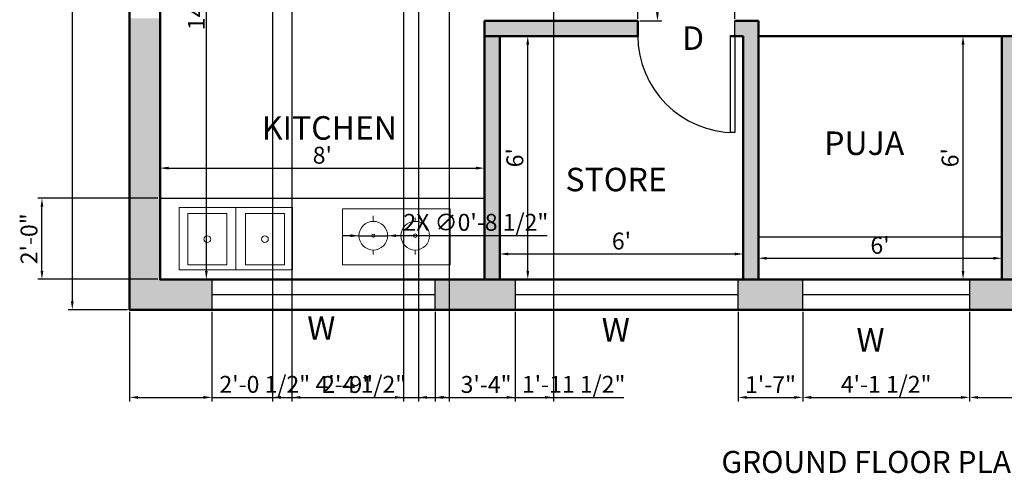
# Model space of a CAD drawing. Units: inches. Extents: x 2168 to 2706, y 2255 to 2760.
# Tile 1 of 4: x 2172 to 2463, y 2255 to 2389. Entities that reach past the tile are written whole.
import ezdxf

# ---------------------------------------------------------------- set-up
doc = ezdxf.new("R2010")
doc.units = ezdxf.units.IN
for name, color, linetype, lineweight in [('A-ANNO-DIMS', 220, 'Continuous', 18), ('A-ANNO-TEXT', 220, 'Continuous', 25), ('A-AREA-IDEN', 220, 'Continuous', 25), ('A-EQPM', 112, 'Continuous', 18), ('A-FLOR-CASE', 112, 'Continuous', 25), ('A-FLOR-FIXT', 9, 'Continuous', 18), ('A-WALL-PATT', 140, 'Continuous', 13), ('DOOR', 30, 'Continuous', 25), ('WALL', 140, 'Continuous', 50), ('WINDOW', 200, 'Continuous', 25)]:
    doc.layers.add(name, color=color, linetype=linetype, lineweight=lineweight)
doc.styles.get("Standard").update_dxf_attribs({"font": 'arial.ttf'})
doc.dimstyles.new('ISO-25', dxfattribs={"dimtxt": 5, "dimasz": 2.5, "dimexe": 1.25, "dimexo": 0.625, "dimtad": 1, "dimlunit": 4, "dimtxsty": 'Standard', "dimcen": 2.5, "dimadec": 0, "dimazin": 0, "dimtfac": 1, "dimtmove": 0, "dimatfit": 3, "dimfxl": 1, "dimarcsym": 0})

# ---------------------------------------------------------------- blocks, each defined once
blk = doc.blocks.new('*U2')
for p, q in [((0, 0), (0, -6)), ((40, 0), (40, -6))]:
    blk.add_line(p, q)
blk.add_lwpolyline([(0, 0), (0, 40), (1.75, 40), (1.75, 0)], close=True)
blk.add_arc((0, 0), 40, 0, 90)
blk = doc.blocks.new('*D11')
at = {"layer": 'A-ANNO-DIMS', "color": 0, "lineweight": -2, "transparency": 16777216}
for p, q in [((2213.72, 2312.97), (2213.72, 2346.52)), ((2216.22, 2345.27), (2307.22, 2345.27)), ((2309.72, 2312.97), (2309.72, 2346.52))]:
    blk.add_line(p, q, dxfattribs=at)
at = {"layer": 'A-ANNO-DIMS', "color": 0, "transparency": 16777216}
for points in [[(2216.22, 2345.69), (2216.22, 2344.85), (2213.72, 2345.27)], [(2307.22, 2345.69), (2307.22, 2344.85), (2309.72, 2345.27)]]:
    blk.add_solid(points, dxfattribs=at)
at = {"layer": 'Defpoints', "color": 0, "transparency": 16777216}
for p in [(2309.72, 2345.27), (2213.72, 2312.35), (2309.72, 2312.35)]:
    blk.add_point(p, dxfattribs=at)
at = {"layer": 'A-ANNO-DIMS', "color": 0, "transparency": 16777216, "insert": (2261.72, 2348.45), "char_height": 5, "attachment_point": 5}
blk.add_mtext("8'", dxfattribs=at)
blk = doc.blocks.new('*D12')
at = {"layer": 'A-ANNO-DIMS', "color": 0, "lineweight": -2, "transparency": 16777216}
for p, q in [((2314.22, 2312.97), (2314.22, 2321.11)), ((2316.72, 2319.86), (2383.72, 2319.86)), ((2386.22, 2312.97), (2386.22, 2321.11))]:
    blk.add_line(p, q, dxfattribs=at)
at = {"layer": 'A-ANNO-DIMS', "color": 0, "transparency": 16777216}
for points in [[(2316.72, 2320.27), (2316.72, 2319.44), (2314.22, 2319.86)], [(2383.72, 2320.27), (2383.72, 2319.44), (2386.22, 2319.86)]]:
    blk.add_solid(points, dxfattribs=at)
at = {"layer": 'Defpoints', "color": 0, "transparency": 16777216}
for p in [(2386.22, 2319.86), (2314.22, 2312.35), (2386.22, 2312.35)]:
    blk.add_point(p, dxfattribs=at)
at = {"layer": 'A-ANNO-DIMS', "color": 0, "transparency": 16777216, "insert": (2350.22, 2323.04), "char_height": 5, "attachment_point": 5}
blk.add_mtext("6'", dxfattribs=at)
blk = doc.blocks.new('*D13')
at = {"layer": 'A-ANNO-DIMS', "color": 0, "lineweight": -2, "transparency": 16777216}
for p, q in [((2390.72, 2312.97), (2390.72, 2319.84)), ((2462.72, 2312.97), (2462.72, 2319.84)), ((2393.22, 2318.59), (2460.22, 2318.59))]:
    blk.add_line(p, q, dxfattribs=at)
at = {"layer": 'A-ANNO-DIMS', "color": 0, "transparency": 16777216}
for points in [[(2393.22, 2319.01), (2393.22, 2318.17), (2390.72, 2318.59)], [(2460.22, 2319.01), (2460.22, 2318.17), (2462.72, 2318.59)]]:
    blk.add_solid(points, dxfattribs=at)
at = {"layer": 'Defpoints', "color": 0, "transparency": 16777216}
for p in [(2462.72, 2318.59), (2390.72, 2312.35), (2462.72, 2312.35)]:
    blk.add_point(p, dxfattribs=at)
at = {"layer": 'A-ANNO-DIMS', "color": 0, "transparency": 16777216, "insert": (2426.72, 2321.77), "char_height": 5, "attachment_point": 5}
blk.add_mtext("6'", dxfattribs=at)
blk = doc.blocks.new('*D24')
at = {"layer": 'A-ANNO-DIMS', "color": 0, "lineweight": -2, "transparency": 16777216}
for p, q in [((2355.67, 2565.85), (2362.12, 2565.85)), ((2360.87, 2391.35), (2360.87, 2563.35)), ((2355.67, 2388.85), (2362.12, 2388.85))]:
    blk.add_line(p, q, dxfattribs=at)
at = {"layer": 'A-ANNO-DIMS', "color": 0, "transparency": 16777216}
for points in [[(2360.45, 2563.35), (2361.28, 2563.35), (2360.87, 2565.85)], [(2360.45, 2391.35), (2361.28, 2391.35), (2360.87, 2388.85)]]:
    blk.add_solid(points, dxfattribs=at)
at = {"layer": 'Defpoints', "color": 0, "transparency": 16777216}
for p in [(2355.04, 2565.85), (2360.87, 2565.85), (2355.04, 2388.85)]:
    blk.add_point(p, dxfattribs=at)
at = {"layer": 'A-ANNO-DIMS', "color": 0, "transparency": 16777216, "insert": (2357.69, 2477.35), "char_height": 5, "attachment_point": 5, "rotation": 90}
blk.add_mtext('14\'-9"', dxfattribs=at)
blk = doc.blocks.new('*D26')
at = {"layer": 'A-ANNO-DIMS', "color": 0, "lineweight": -2, "transparency": 16777216}
for p, q in [((2462.1, 2384.35), (2450.03, 2384.35)), ((2451.28, 2314.85), (2451.28, 2381.85)), ((2462.1, 2312.35), (2450.03, 2312.35))]:
    blk.add_line(p, q, dxfattribs=at)
at = {"layer": 'A-ANNO-DIMS', "color": 0, "transparency": 16777216}
for points in [[(2450.87, 2381.85), (2451.7, 2381.85), (2451.28, 2384.35)], [(2450.87, 2314.85), (2451.7, 2314.85), (2451.28, 2312.35)]]:
    blk.add_solid(points, dxfattribs=at)
at = {"layer": 'Defpoints', "color": 0, "transparency": 16777216}
for p in [(2451.28, 2384.35), (2462.72, 2384.35), (2462.72, 2312.35)]:
    blk.add_point(p, dxfattribs=at)
at = {"layer": 'A-ANNO-DIMS', "color": 0, "transparency": 16777216, "insert": (2448.1, 2348.35), "char_height": 5, "attachment_point": 5, "rotation": 90}
blk.add_mtext("6'", dxfattribs=at)
blk = doc.blocks.new('*D27')
at = {"layer": 'A-ANNO-DIMS', "color": 0, "lineweight": -2, "transparency": 16777216}
for p, q in [((2314.85, 2384.35), (2323.75, 2384.35)), ((2322.5, 2314.85), (2322.5, 2381.85)), ((2314.85, 2312.35), (2323.75, 2312.35))]:
    blk.add_line(p, q, dxfattribs=at)
at = {"layer": 'A-ANNO-DIMS', "color": 0, "transparency": 16777216}
for points in [[(2322.09, 2381.85), (2322.92, 2381.85), (2322.5, 2384.35)], [(2322.09, 2314.85), (2322.92, 2314.85), (2322.5, 2312.35)]]:
    blk.add_solid(points, dxfattribs=at)
at = {"layer": 'Defpoints', "color": 0, "transparency": 16777216}
for p in [(2314.22, 2384.35), (2322.5, 2384.35), (2314.22, 2312.35)]:
    blk.add_point(p, dxfattribs=at)
at = {"layer": 'A-ANNO-DIMS', "color": 0, "transparency": 16777216, "insert": (2319.33, 2348.35), "char_height": 5, "attachment_point": 5, "rotation": 90}
blk.add_mtext("6'", dxfattribs=at)
blk = doc.blocks.new('*D28')
at = {"layer": 'A-ANNO-DIMS', "color": 0, "lineweight": -2, "transparency": 16777216}
for p, q in [((2214.35, 2482.49), (2228.66, 2482.49)), ((2227.41, 2314.85), (2227.41, 2479.99)), ((2214.35, 2312.35), (2228.66, 2312.35))]:
    blk.add_line(p, q, dxfattribs=at)
at = {"layer": 'A-ANNO-DIMS', "color": 0, "transparency": 16777216}
for points in [[(2227, 2479.99), (2227.83, 2479.99), (2227.41, 2482.49)], [(2227, 2314.85), (2227.83, 2314.85), (2227.41, 2312.35)]]:
    blk.add_solid(points, dxfattribs=at)
at = {"layer": 'Defpoints', "color": 0, "transparency": 16777216}
for p in [(2213.72, 2482.49), (2227.41, 2482.49), (2213.72, 2312.35)]:
    blk.add_point(p, dxfattribs=at)
at = {"layer": 'A-ANNO-DIMS', "color": 0, "transparency": 16777216, "insert": (2220.94, 2397.42), "char_height": 5, "attachment_point": 5, "rotation": 90}
blk.add_mtext('14\'-2{\\H1x;\\S1/4;}"', dxfattribs=at)
blk = doc.blocks.new('*D30')
at = {"layer": 'A-ANNO-DIMS', "color": 0, "lineweight": -2, "transparency": 16777216}
for p, q in [((2204.1, 2723.35), (2186.49, 2723.35)), ((2187.74, 2720.85), (2187.74, 2305.85)), ((2204.1, 2303.35), (2186.49, 2303.35))]:
    blk.add_line(p, q, dxfattribs=at)
at = {"layer": 'A-ANNO-DIMS', "color": 0, "transparency": 16777216}
for points in [[(2187.33, 2720.85), (2188.16, 2720.85), (2187.74, 2723.35)], [(2187.33, 2305.85), (2188.16, 2305.85), (2187.74, 2303.35)]]:
    blk.add_solid(points, dxfattribs=at)
at = {"layer": 'Defpoints', "color": 0, "transparency": 16777216}
for p in [(2204.72, 2723.35), (2187.74, 2303.35), (2204.72, 2303.35)]:
    blk.add_point(p, dxfattribs=at)
at = {"layer": 'A-ANNO-DIMS', "color": 0, "transparency": 16777216, "insert": (2184.56, 2513.35), "char_height": 5, "attachment_point": 5, "rotation": 90}
blk.add_mtext("35'", dxfattribs=at)
blk = doc.blocks.new('WIN-66IN')
blk.add_line((0, 0), (66.01, 0))
blk.add_lwpolyline([(0, -4.5), (66.01, -4.5), (66.01, 4.5), (0, 4.5)], close=True)
blk = doc.blocks.new('*D49')
at = {"layer": 'A-ANNO-DIMS', "color": 0, "lineweight": -2, "transparency": 16777216}
for p, q in [((2355.04, 2389.47), (2355.04, 2750.55)), ((2383.78, 2389.47), (2383.78, 2750.55)), ((2357.54, 2749.3), (2381.28, 2749.3))]:
    blk.add_line(p, q, dxfattribs=at)
at = {"layer": 'A-ANNO-DIMS', "color": 0, "transparency": 16777216}
for points in [[(2357.54, 2749.71), (2357.54, 2748.88), (2355.04, 2749.3)], [(2381.28, 2749.71), (2381.28, 2748.88), (2383.78, 2749.3)]]:
    blk.add_solid(points, dxfattribs=at)
at = {"layer": 'Defpoints', "color": 0, "transparency": 16777216}
for p in [(2383.78, 2749.3), (2355.04, 2388.85), (2383.78, 2388.85)]:
    blk.add_point(p, dxfattribs=at)
at = {"layer": 'A-ANNO-DIMS', "color": 0, "transparency": 16777216, "insert": (2369.41, 2752.51), "char_height": 5, "attachment_point": 5}
blk.add_mtext('2\'-4 1/2"', dxfattribs=at)
blk = doc.blocks.new('*D54')
at = {"layer": 'A-ANNO-DIMS', "color": 0, "lineweight": -2, "transparency": 16777216}
for p, q in [((2246.96, 2425.79), (2246.96, 2276.15)), ((2299.27, 2425.79), (2299.27, 2276.15)), ((2249.46, 2277.4), (2296.77, 2277.4))]:
    blk.add_line(p, q, dxfattribs=at)
at = {"layer": 'A-ANNO-DIMS', "color": 0, "transparency": 16777216}
for points in [[(2249.46, 2277.81), (2249.46, 2276.98), (2246.96, 2277.4)], [(2296.77, 2277.81), (2296.77, 2276.98), (2299.27, 2277.4)]]:
    blk.add_solid(points, dxfattribs=at)
at = {"layer": 'Defpoints', "color": 0, "transparency": 16777216}
for p in [(2246.96, 2426.42), (2299.27, 2426.42), (2299.27, 2277.4)]:
    blk.add_point(p, dxfattribs=at)
at = {"layer": 'A-ANNO-DIMS', "color": 0, "transparency": 16777216, "insert": (2273.11, 2280.61), "char_height": 5, "attachment_point": 5}
blk.add_mtext('4\'-4 1/2"', dxfattribs=at)
blk = doc.blocks.new('*D56')
at = {"layer": 'A-ANNO-DIMS', "color": 0, "lineweight": -2, "transparency": 16777216}
for p, q in [((2213.1, 2336.35), (2177.52, 2336.35)), ((2178.77, 2314.85), (2178.77, 2333.85)), ((2213.1, 2312.35), (2177.52, 2312.35))]:
    blk.add_line(p, q, dxfattribs=at)
at = {"layer": 'A-ANNO-DIMS', "color": 0, "transparency": 16777216}
for points in [[(2178.36, 2333.85), (2179.19, 2333.85), (2178.77, 2336.35)], [(2178.36, 2314.85), (2179.19, 2314.85), (2178.77, 2312.35)]]:
    blk.add_solid(points, dxfattribs=at)
at = {"layer": 'Defpoints', "color": 0, "transparency": 16777216}
for p in [(2178.77, 2336.35), (2213.72, 2336.35), (2213.72, 2312.35)]:
    blk.add_point(p, dxfattribs=at)
at = {"layer": 'A-ANNO-DIMS', "color": 0, "transparency": 16777216, "insert": (2175.6, 2324.35), "char_height": 5, "attachment_point": 5, "rotation": 90}
blk.add_mtext('2\'-0"', dxfattribs=at)
blk = doc.blocks.new('*D57')
at = {"layer": 'A-ANNO-DIMS', "color": 0, "lineweight": -2, "transparency": 16777216}
for p, q in [((2204.72, 2302.72), (2204.72, 2276.15)), ((2229.06, 2302.72), (2229.06, 2276.15)), ((2207.22, 2277.4), (2226.56, 2277.4)), ((2229.06, 2277.4), (2257.84, 2277.4))]:
    blk.add_line(p, q, dxfattribs=at)
at = {"layer": 'A-ANNO-DIMS', "color": 0, "transparency": 16777216}
for points in [[(2207.22, 2277.81), (2207.22, 2276.98), (2204.72, 2277.4)], [(2226.56, 2277.81), (2226.56, 2276.98), (2229.06, 2277.4)]]:
    blk.add_solid(points, dxfattribs=at)
at = {"layer": 'Defpoints', "color": 0, "transparency": 16777216}
for p in [(2204.72, 2303.35), (2229.06, 2303.35), (2229.06, 2277.4)]:
    blk.add_point(p, dxfattribs=at)
at = {"layer": 'A-ANNO-DIMS', "color": 0, "transparency": 16777216, "insert": (2244.7, 2280.61), "char_height": 5, "attachment_point": 5}
blk.add_mtext('2\'-0 1/2"', dxfattribs=at)
blk = doc.blocks.new('*D58')
at = {"layer": 'A-ANNO-DIMS', "color": 0, "lineweight": -2, "transparency": 16777216}
for p, q in [((2295.07, 2302.72), (2295.07, 2276.15)), ((2318.77, 2302.72), (2318.77, 2276.15)), ((2297.57, 2277.4), (2316.27, 2277.4)), ((2318.77, 2277.4), (2350.88, 2277.4))]:
    blk.add_line(p, q, dxfattribs=at)
at = {"layer": 'A-ANNO-DIMS', "color": 0, "transparency": 16777216}
for points in [[(2297.57, 2277.81), (2297.57, 2276.98), (2295.07, 2277.4)], [(2316.27, 2277.81), (2316.27, 2276.98), (2318.77, 2277.4)]]:
    blk.add_solid(points, dxfattribs=at)
at = {"layer": 'Defpoints', "color": 0, "transparency": 16777216}
for p in [(2295.07, 2303.35), (2318.77, 2303.35), (2318.77, 2277.4)]:
    blk.add_point(p, dxfattribs=at)
at = {"layer": 'A-ANNO-DIMS', "color": 0, "transparency": 16777216, "insert": (2336.08, 2280.61), "char_height": 5, "attachment_point": 5}
blk.add_mtext('1\'-11 1/2"', dxfattribs=at)
blk = doc.blocks.new('*D59')
at = {"layer": 'A-ANNO-DIMS', "color": 0, "lineweight": -2, "transparency": 16777216}
for p, q in [((2384.78, 2302.72), (2384.78, 2276.15)), ((2403.85, 2302.72), (2403.85, 2276.15)), ((2387.28, 2277.4), (2401.35, 2277.4))]:
    blk.add_line(p, q, dxfattribs=at)
at = {"layer": 'A-ANNO-DIMS', "color": 0, "transparency": 16777216}
for points in [[(2387.28, 2277.81), (2387.28, 2276.98), (2384.78, 2277.4)], [(2401.35, 2277.81), (2401.35, 2276.98), (2403.85, 2277.4)]]:
    blk.add_solid(points, dxfattribs=at)
at = {"layer": 'Defpoints', "color": 0, "transparency": 16777216}
for p in [(2384.78, 2303.35), (2403.85, 2303.35), (2403.85, 2277.4)]:
    blk.add_point(p, dxfattribs=at)
at = {"layer": 'A-ANNO-DIMS', "color": 0, "transparency": 16777216, "insert": (2394.32, 2280.53), "char_height": 5, "attachment_point": 5}
blk.add_mtext('1\'-7"', dxfattribs=at)
blk = doc.blocks.new('*D60')
at = {"layer": 'A-ANNO-DIMS', "color": 0, "lineweight": -2, "transparency": 16777216}
for p, q in [((2403.85, 2302.72), (2403.85, 2276.15)), ((2453.21, 2302.72), (2453.21, 2276.15)), ((2406.35, 2277.4), (2450.71, 2277.4))]:
    blk.add_line(p, q, dxfattribs=at)
at = {"layer": 'A-ANNO-DIMS', "color": 0, "transparency": 16777216}
for points in [[(2406.35, 2277.81), (2406.35, 2276.98), (2403.85, 2277.4)], [(2450.71, 2277.81), (2450.71, 2276.98), (2453.21, 2277.4)]]:
    blk.add_solid(points, dxfattribs=at)
at = {"layer": 'Defpoints', "color": 0, "transparency": 16777216}
for p in [(2403.85, 2303.35), (2453.21, 2303.35), (2453.21, 2277.4)]:
    blk.add_point(p, dxfattribs=at)
at = {"layer": 'A-ANNO-DIMS', "color": 0, "transparency": 16777216, "insert": (2428.53, 2280.61), "char_height": 5, "attachment_point": 5}
blk.add_mtext('4\'-1 1/2"', dxfattribs=at)
blk = doc.blocks.new('*D61')
at = {"layer": 'A-ANNO-DIMS', "color": 0, "lineweight": -2, "transparency": 16777216}
for p, q in [((2453.21, 2302.72), (2453.21, 2276.15)), ((2493.42, 2302.72), (2493.42, 2276.15)), ((2455.71, 2277.4), (2490.92, 2277.4))]:
    blk.add_line(p, q, dxfattribs=at)
at = {"layer": 'A-ANNO-DIMS', "color": 0, "transparency": 16777216}
for points in [[(2455.71, 2277.81), (2455.71, 2276.98), (2453.21, 2277.4)], [(2490.92, 2277.81), (2490.92, 2276.98), (2493.42, 2277.4)]]:
    blk.add_solid(points, dxfattribs=at)
at = {"layer": 'Defpoints', "color": 0, "transparency": 16777216}
for p in [(2453.21, 2303.35), (2493.42, 2303.35), (2493.42, 2277.4)]:
    blk.add_point(p, dxfattribs=at)
at = {"layer": 'A-ANNO-DIMS', "color": 0, "transparency": 16777216, "insert": (2473.31, 2280.58), "char_height": 5, "attachment_point": 5}
blk.add_mtext('3\'-4"', dxfattribs=at)
blk = doc.blocks.new('*D64')
at = {"layer": 'A-ANNO-DIMS', "color": 0, "lineweight": -2, "transparency": 16777216}
for p, q in [((2290.22, 2713.72), (2290.22, 2276.15)), ((2330.12, 2713.72), (2330.12, 2276.15)), ((2292.72, 2277.4), (2327.62, 2277.4))]:
    blk.add_line(p, q, dxfattribs=at)
at = {"layer": 'A-ANNO-DIMS', "color": 0, "transparency": 16777216}
for points in [[(2292.72, 2277.81), (2292.72, 2276.98), (2290.22, 2277.4)], [(2327.62, 2277.81), (2327.62, 2276.98), (2330.12, 2277.4)]]:
    blk.add_solid(points, dxfattribs=at)
at = {"layer": 'Defpoints', "color": 0, "transparency": 16777216}
for p in [(2290.22, 2714.35), (2330.12, 2714.35), (2330.12, 2277.4)]:
    blk.add_point(p, dxfattribs=at)
at = {"layer": 'A-ANNO-DIMS', "color": 0, "transparency": 16777216, "insert": (2310.17, 2280.58), "char_height": 5, "attachment_point": 5}
blk.add_mtext('3\'-4"', dxfattribs=at)
blk = doc.blocks.new('*D76')
at = {"layer": 'A-ANNO-DIMS', "color": 0, "lineweight": -2, "transparency": 16777216}
for p, q in [((2252.72, 2623.46), (2252.72, 2276.15)), ((2285.72, 2612.95), (2285.72, 2276.15)), ((2255.22, 2277.4), (2283.22, 2277.4))]:
    blk.add_line(p, q, dxfattribs=at)
at = {"layer": 'A-ANNO-DIMS', "color": 0, "transparency": 16777216}
for points in [[(2255.22, 2277.81), (2255.22, 2276.98), (2252.72, 2277.4)], [(2283.22, 2277.81), (2283.22, 2276.98), (2285.72, 2277.4)]]:
    blk.add_solid(points, dxfattribs=at)
at = {"layer": 'Defpoints', "color": 0, "transparency": 16777216}
for p in [(2252.72, 2624.08), (2285.72, 2613.58), (2285.72, 2277.4)]:
    blk.add_point(p, dxfattribs=at)
at = {"layer": 'A-ANNO-DIMS', "color": 0, "transparency": 16777216, "insert": (2269.22, 2280.57), "char_height": 5, "attachment_point": 5}
blk.add_mtext('2\'-9"', dxfattribs=at)
blk = doc.blocks.new('*D78')
at = {"layer": 'A-ANNO-DIMS', "color": 0, "lineweight": -2, "transparency": 16777216}
for p, q in [((2270.05, 2325.26), (2267.55, 2325.26)), ((2272.55, 2325.26), (2281.04, 2325.26)), ((2328.24, 2325.26), (2283.54, 2325.26))]:
    blk.add_line(p, q, dxfattribs=at)
at = {"layer": 'A-ANNO-DIMS', "color": 0, "transparency": 16777216}
for points in [[(2270.05, 2325.68), (2270.05, 2324.84), (2272.55, 2325.26)], [(2283.54, 2325.68), (2283.54, 2324.84), (2281.04, 2325.26)]]:
    blk.add_solid(points, dxfattribs=at)
at = {"layer": 'Defpoints', "color": 0, "transparency": 16777216}
for p in [(2272.55, 2325.26), (2281.04, 2325.26)]:
    blk.add_point(p, dxfattribs=at)
at = {"layer": 'A-ANNO-DIMS', "color": 0, "transparency": 16777216, "insert": (2307.14, 2328.58), "char_height": 5, "attachment_point": 5, "rotation": 359.9965}
blk.add_mtext('2X ∅0\'-8 1/2"', dxfattribs=at)

msp = doc.modelspace()

# ---------------------------------------------------------------- hatches: boundary and pattern name
at = {"layer": 'A-WALL-PATT'}
h = msp.add_hatch(color=256, dxfattribs=at)
h.dxf.hatch_style = 1
h.paths.add_polyline_path([(2330.12, 2723.347), (2204.724, 2723.347), (2204.724, 2662.147), (2213.724, 2662.147), (2213.724, 2714.347), (2285.724, 2714.347), (2330.12, 2714.347)])
h.paths.add_polyline_path([(2496.542, 2723.347), (2396.128, 2723.347), (2396.128, 2714.347), (2434.224, 2714.347), (2496.542, 2714.347)])
h.paths.add_polyline_path([(2624.724, 2723.347), (2562.55, 2723.347), (2562.55, 2714.347), (2615.724, 2714.347), (2615.724, 2545.448), (2624.724, 2545.448)])
h.paths.add_polyline_path([(2438.724, 2714.347), (2434.224, 2714.347), (2434.224, 2570.347), (2426.591, 2570.347), (2426.591, 2565.847), (2438.724, 2565.847), (2444.149, 2565.847), (2444.149, 2570.347), (2438.724, 2570.347)])
h.paths.add_polyline_path([(2290.224, 2668.023), (2285.724, 2668.023), (2285.724, 2570.347), (2213.724, 2570.347), (2213.724, 2565.847), (2290.224, 2565.847), (2386.591, 2565.847), (2386.591, 2570.347), (2290.224, 2570.347)])
h.paths.add_polyline_path([(2514.678, 2570.347), (2514.678, 2630.11), (2560.439, 2630.11), (2560.439, 2570.347)], flags=16)
h.paths.add_polyline_path([(2517.528, 2574.595), (2517.528, 2583.399), (2536.063, 2583.399), (2536.063, 2574.595)], flags=0)
h.paths.add_polyline_path([(2523.909, 2586.89), (2514.678, 2597.212), (2518.822, 2600.918)], flags=0)
h.paths.add_polyline_path([(2538.189, 2574.595), (2538.189, 2583.399), (2556.724, 2583.399), (2556.724, 2574.595)], flags=0)
h.paths.add_polyline_path([(2560.439, 2630.11), (2560.439, 2570.347), (2514.678, 2570.347), (2514.678, 2630.11)])
h.paths.add_polyline_path([(2213.724, 2389.588), (2204.724, 2389.588), (2204.724, 2303.347), (2229.06, 2303.347), (2229.06, 2312.347), (2213.724, 2312.347)])
h.paths.add_polyline_path([(2213.724, 2507.677), (2204.724, 2507.677), (2204.724, 2462.696), (2213.724, 2462.696)])
h.paths.add_polyline_path([(2204.724, 2553.759), (2213.724, 2553.759), (2213.724, 2613.731), (2204.724, 2613.731)])
h = msp.add_hatch(color=256, dxfattribs=at)
h.dxf.hatch_style = 1
h.paths.add_polyline_path([(2318.775, 2312.347), (2295.068, 2312.347), (2295.068, 2303.347), (2318.775, 2303.347)])
h.paths.add_polyline_path([(2403.851, 2312.347), (2390.724, 2312.347), (2384.782, 2312.347), (2384.782, 2303.347), (2403.851, 2303.347)])
h.paths.add_polyline_path([(2390.724, 2384.347), (2390.724, 2388.847), (2383.783, 2388.847), (2383.783, 2384.347), (2386.224, 2384.347), (2386.224, 2312.347), (2390.724, 2312.347), (2390.724, 2324.834)])
h.paths.add_polyline_path([(2493.418, 2312.347), (2467.224, 2312.347), (2453.211, 2312.347), (2453.211, 2303.347), (2493.418, 2303.347)])
h.paths.add_polyline_path([(2467.224, 2384.347), (2462.724, 2384.347), (2462.724, 2312.347), (2467.224, 2312.347)])
h.paths.add_polyline_path([(2572.054, 2309.347, -0.0187698), (2572.166, 2312.347), (2562.881, 2312.347), (2562.881, 2303.347), (2572.054, 2303.347)])
h.paths.add_polyline_path([(2624.724, 2433.98), (2615.724, 2433.98), (2615.724, 2432.059), (2615.724, 2412.847), (2615.724, 2312.347), (2612.054, 2312.347), (2612.054, 2309.347), (2612.054, 2303.347), (2624.724, 2303.347)])
h.paths.add_polyline_path([(2543.724, 2452.016), (2543.724, 2458.843, -0.0148288), (2542.449, 2458.805), (2539.224, 2458.805), (2539.224, 2452.016), (2539.224, 2412.847), (2543.724, 2412.847)])
h.paths.add_polyline_path([(2615.724, 2412.847), (2543.724, 2412.847), (2539.224, 2412.847), (2539.224, 2408.347), (2615.724, 2408.347)])
h.paths.add_polyline_path([(2624.724, 2513.509), (2615.724, 2513.509), (2615.724, 2465.92), (2624.724, 2465.92)])
h.paths.add_polyline_path([(2588.15, 2570.347), (2484.149, 2570.347), (2484.149, 2565.847), (2588.176, 2565.847, -0.0118396), (2588.15, 2566.926)])
h.paths.add_polyline_path([(2615.724, 2570.347), (2610.953, 2570.347), (2610.953, 2566.926), (2610.953, 2565.847), (2615.724, 2565.847)])
h.paths.add_polyline_path([(2519.724, 2565.847), (2515.224, 2565.847), (2515.224, 2489.347), (2519.724, 2489.347)])
h.paths.add_polyline_path([(2615.724, 2489.347), (2519.724, 2489.347), (2515.224, 2489.347), (2515.224, 2484.847), (2615.724, 2484.847)])
h.paths.add_polyline_path([(2543.724, 2484.847), (2539.224, 2484.847), (2539.224, 2480.308), (2542.449, 2480.308), (2543.724, 2480.308)])
h = msp.add_hatch(color=256, dxfattribs=at)
h.dxf.hatch_style = 1
h.paths.add_polyline_path([(2355.045, 2388.847), (2309.724, 2388.847), (2309.724, 2384.347), (2355.045, 2384.347)])
h.paths.add_polyline_path([(2314.224, 2384.347), (2309.724, 2384.347), (2309.724, 2312.347), (2314.224, 2312.347)])

# ---------------------------------------------------------------- linework, layer by layer
at = {"layer": 'A-EQPM'}
for p, q in [((2276.797, 2329.507), (2276.797, 2331.145)), ((2289.211, 2329.507), (2289.211, 2330.653)), ((2272.55, 2325.26), (2271.409, 2325.26)), ((2281.044, 2325.26), (2282.085, 2325.26)), ((2284.965, 2325.26), (2283.529, 2325.26)), ((2293.458, 2325.26), (2294.789, 2325.26)), ((2276.797, 2321.013), (2276.797, 2319.71)), ((2289.211, 2321.013), (2289.211, 2319.701))]:
    msp.add_line(p, q, dxfattribs=at)
msp.add_lwpolyline([(2267.741, 2316.632), (2299.532, 2316.632), (2299.532, 2333.255), (2267.741, 2333.255)], close=True, dxfattribs=at)
for centre, radius in [((2276.797, 2325.26), 4.247), ((2289.211, 2325.26), 4.247), ((2276.797, 2325.26), 0.467), ((2289.211, 2325.26), 0.516)]:
    msp.add_circle(centre, radius, dxfattribs=at)
at = {"layer": 'A-FLOR-CASE'}
for p, q in [((2213.724, 2312.347), (2213.724, 2336.347)), ((2213.724, 2336.347), (2309.724, 2336.347))]:
    msp.add_line(p, q, dxfattribs=at)
msp.add_lwpolyline([(2390.724, 2312.347), (2462.724, 2312.347), (2462.724, 2324.834), (2390.724, 2324.834)], close=True, dxfattribs=at)
at = {"layer": 'A-FLOR-FIXT'}
msp.add_line((2236.163, 2315.158), (2236.163, 2333.657), dxfattribs=at)
for points in [[(2219.383, 2315.158), (2252.942, 2315.158), (2252.942, 2333.657), (2219.383, 2333.657)], [(2221.908, 2316.63), (2233.48, 2316.63), (2233.48, 2331.87), (2221.908, 2331.87)], [(2238.95, 2316.63), (2250.523, 2316.63), (2250.523, 2331.87), (2238.95, 2331.87)]]:
    msp.add_lwpolyline(points, close=True, dxfattribs=at)
for centre in [(2227.694, 2324.25), (2244.737, 2324.25)]:
    msp.add_circle(centre, 0.999, dxfattribs=at)
at = {"layer": 'WALL'}
for p, q in [((2204.724, 2303.347), (2204.724, 2723.347)), ((2309.724, 2312.347), (2309.724, 2388.847)), ((2355.045, 2388.847), (2309.724, 2388.847)), ((2390.724, 2388.847), (2383.783, 2388.847)), ((2390.724, 2312.347), (2390.724, 2388.847)), ((2314.224, 2312.347), (2314.224, 2384.347)), ((2355.045, 2384.347), (2314.224, 2384.347)), ((2386.224, 2384.347), (2382.525, 2384.347)), ((2386.224, 2312.347), (2386.224, 2384.347)), ((2390.724, 2312.347), (2390.724, 2384.347)), ((2390.724, 2384.347), (2462.724, 2384.347)), ((2462.724, 2384.347), (2462.724, 2312.347)), ((2462.724, 2384.347), (2467.224, 2384.347)), ((2213.724, 2312.347), (2309.724, 2312.347)), ((2314.224, 2312.347), (2386.224, 2312.347)), ((2572.054, 2303.347), (2204.724, 2303.347))]:
    msp.add_line(p, q, dxfattribs=at)
for points in [[(2572.054, 2303.347), (2204.724, 2303.347), (2204.724, 2723.347), (2624.724, 2723.347), (2624.724, 2303.347), (2612.054, 2303.347)], [(2572.166, 2312.347), (2213.724, 2312.347), (2213.724, 2714.347), (2615.724, 2714.347), (2615.724, 2312.347), (2610.304, 2312.347)]]:
    msp.add_lwpolyline(points, dxfattribs=at)
for points in [[(2309.724, 2384.347), (2355.045, 2384.347), (2355.045, 2388.847), (2309.724, 2388.847)], [(2309.724, 2312.347), (2314.224, 2312.347), (2314.224, 2384.347), (2309.724, 2384.347)]]:
    msp.add_lwpolyline(points, close=True, dxfattribs=at)
at = {"layer": 'WINDOW'}
msp.add_line((2403.851, 2307.847), (2453.211, 2307.847), dxfattribs=at)
msp.add_lwpolyline([(2403.851, 2312.347), (2453.211, 2312.347), (2453.211, 2303.347), (2403.851, 2303.347)], close=True, dxfattribs=at)

# ---------------------------------------------------------------- block references
at = {"layer": 'DOOR', "xscale": 0.7184482752319159, "yscale": 0.7184482752319159, "zscale": 0.7184482752319159, "rotation": 180}
msp.add_blockref('*U2', (2383.783, 2384.536), dxfattribs=at)
at = {"layer": 'WINDOW'}
for p in [(2229.06, 2307.847), (2318.775, 2307.847)]:
    msp.add_blockref('WIN-66IN', p, dxfattribs=at)

# ---------------------------------------------------------------- texts
at = {"layer": 'A-ANNO-TEXT', "attachment_point": 1}
for s, width, gutter_width, insert, char_height in [('D', 121.01281, 34.753, (2368.146, 2387.23), 6.951), ('W', 121.01281, 34.753, (2257.257, 2301.418), 6.951), ('W', 121.01281, 34.753, (2344.379, 2300.878), 6.951), ('W', 121.01281, 34.753, (2419.742, 2297.922), 6.951), ('GROUND FLOOR PLAN', 655.2644, 32.568, (2379.787, 2261.546), 6.51363)]:
    msp.add_mtext_dynamic_manual_height_columns(s, width=width, gutter_width=gutter_width, heights=[0], dxfattribs=dict(at, insert=insert, char_height=char_height))
at = {"layer": 'A-AREA-IDEN', "char_height": 6.9506, "attachment_point": 1}
for s, insert in [('KITCHEN', (2243.854, 2360.645)), ('PUJA', (2410.208, 2356.123)), ('STORE', (2333.67, 2345.364))]:
    msp.add_mtext_dynamic_manual_height_columns(s, width=121.01281, gutter_width=34.753, heights=[0], dxfattribs=dict(at, insert=insert))

# ---------------------------------------------------------------- dimensions: what is measured, and where the dimension line sits
at = {"layer": 'A-ANNO-DIMS'}
for base, p1, p2, override, picture, middle in [((2383.783, 2749.297), (2355.045, 2388.847), (2383.783, 2388.847), {"dimdec": 1, "dimlfac": 1, "dimrnd": 0, "dimzin": 1, "dimdsep": 46, "dimlunit": 4, "dimfrac": 2}, '*D49', (2369.414, 2752.507)), ((2330.12, 2277.397), (2290.224, 2714.347), (2330.12, 2714.347), {"dimdec": 1, "dimlfac": 1, "dimrnd": 0, "dimzin": 1, "dimdsep": 46, "dimlunit": 4, "dimfrac": 2}, '*D64', (2310.172, 2280.577)), ((2285.724, 2277.397), (2252.724, 2624.08), (2285.724, 2613.58), {"dimdec": 1, "dimlfac": 1, "dimrnd": 0, "dimzin": 1, "dimdsep": 46, "dimlunit": 4, "dimfrac": 2}, '*D76', (2269.224, 2280.575)), ((2299.272, 2277.397), (2246.955, 2426.417), (2299.272, 2426.417), {"dimdec": 1, "dimlfac": 1, "dimrnd": 0, "dimzin": 1, "dimdsep": 46, "dimlunit": 4, "dimfrac": 2}, '*D54', (2273.114, 2280.607)), ((2309.724, 2345.27), (2213.724, 2312.347), (2309.724, 2312.347), {"dimclrd": 0, "dimclre": 0, "dimclrt": 0}, '*D11', (2261.724, 2348.448)), ((2386.224, 2319.858), (2314.224, 2312.347), (2386.224, 2312.347), {"dimclrd": 0, "dimclre": 0, "dimclrt": 0}, '*D12', (2350.224, 2323.035)), ((2462.724, 2318.59), (2390.724, 2312.347), (2462.724, 2312.347), {"dimclrd": 0, "dimclre": 0, "dimclrt": 0}, '*D13', (2426.724, 2321.768)), ((2229.06, 2277.397), (2204.724, 2303.347), (2229.06, 2303.347), {"dimdec": 1, "dimlfac": 1, "dimrnd": 0, "dimzin": 1, "dimdsep": 46, "dimlunit": 4, "dimfrac": 2}, '*D57', (2244.699, 2280.607)), ((2318.775, 2277.397), (2295.068, 2303.347), (2318.775, 2303.347), {"dimdec": 1, "dimlfac": 1, "dimrnd": 0, "dimzin": 1, "dimdsep": 46, "dimlunit": 4, "dimfrac": 2}, '*D58', (2336.078, 2280.607)), ((2403.851, 2277.397), (2384.782, 2303.347), (2403.851, 2303.347), {"dimdec": 1, "dimlfac": 1, "dimrnd": 0, "dimzin": 1, "dimdsep": 46, "dimlunit": 4, "dimfrac": 2}, '*D59', (2394.317, 2280.532)), ((2453.211, 2277.397), (2403.851, 2303.347), (2453.211, 2303.347), {"dimdec": 1, "dimlfac": 1, "dimrnd": 0, "dimzin": 1, "dimdsep": 46, "dimlunit": 4, "dimfrac": 2}, '*D60', (2428.531, 2280.607)), ((2493.418, 2277.397), (2453.211, 2303.347), (2493.418, 2303.347), {"dimdec": 1, "dimlfac": 1, "dimrnd": 0, "dimzin": 1, "dimdsep": 46, "dimlunit": 4, "dimfrac": 2}, '*D61', (2473.315, 2280.577))]:
    dim = msp.add_linear_dim(base=base, p1=p1, p2=p2, dimstyle='ISO-25', override=override, dxfattribs=at)
    dim.commit()
    dim.dimension.update_dxf_attribs({"geometry": picture, "text_midpoint": middle})
for base, p1, p2, override, picture, middle in [((2187.744, 2303.347), (2204.724, 2723.347), (2204.724, 2303.347), {"dimclrd": 0, "dimclre": 0, "dimclrt": 0}, '*D30', (2184.565, 2513.347)), ((2360.867, 2565.847), (2355.045, 2388.847), (2355.045, 2565.847), {"dimclrd": 0, "dimclre": 0, "dimclrt": 0}, '*D24', (2357.69, 2477.347)), ((2227.413, 2482.487), (2213.724, 2312.347), (2213.724, 2482.487), {"dimclrd": 0, "dimclre": 0, "dimclrt": 0}, '*D28', (2220.944, 2397.417)), ((2322.505, 2384.347), (2314.224, 2312.347), (2314.224, 2384.347), {"dimclrd": 0, "dimclre": 0, "dimclrt": 0}, '*D27', (2319.327, 2348.347)), ((2451.282, 2384.347), (2462.724, 2312.347), (2462.724, 2384.347), {"dimclrd": 0, "dimclre": 0, "dimclrt": 0}, '*D26', (2448.104, 2348.347)), ((2178.774, 2336.347), (2213.724, 2312.347), (2213.724, 2336.347), {"dimdec": 1, "dimlfac": 1, "dimrnd": 0, "dimzin": 1, "dimdsep": 46, "dimlunit": 4, "dimfrac": 2}, '*D56', (2175.596, 2324.347))]:
    dim = msp.add_linear_dim(base=base, p1=p1, p2=p2, angle=90, dimstyle='ISO-25', override=override, dxfattribs=at)
    dim.commit()
    dim.dimension.update_dxf_attribs({"geometry": picture, "text_midpoint": middle})
dim = msp.add_diameter_dim_2p(p1=(2272.55, 2325.261), p2=(2281.044, 2325.26), text='2X <>', dimstyle='ISO-25', override={"dimdec": 1, "dimlfac": 1, "dimrnd": 0, "dimzin": 1, "dimdsep": 46, "dimlunit": 4, "dimfrac": 2}, dxfattribs=at)
dim.commit()
dim.dimension.update_dxf_attribs({"geometry": '*D78', "text_midpoint": (2307.141, 2325.258)})

doc.saveas('drawing.dxf')
